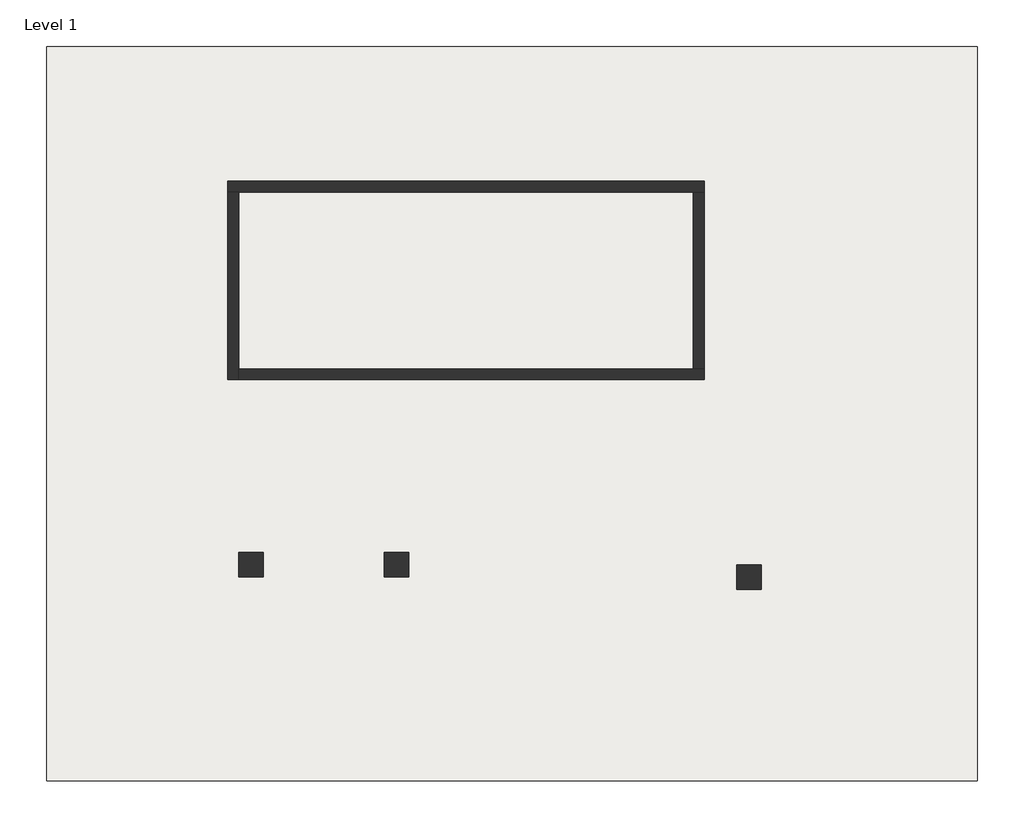
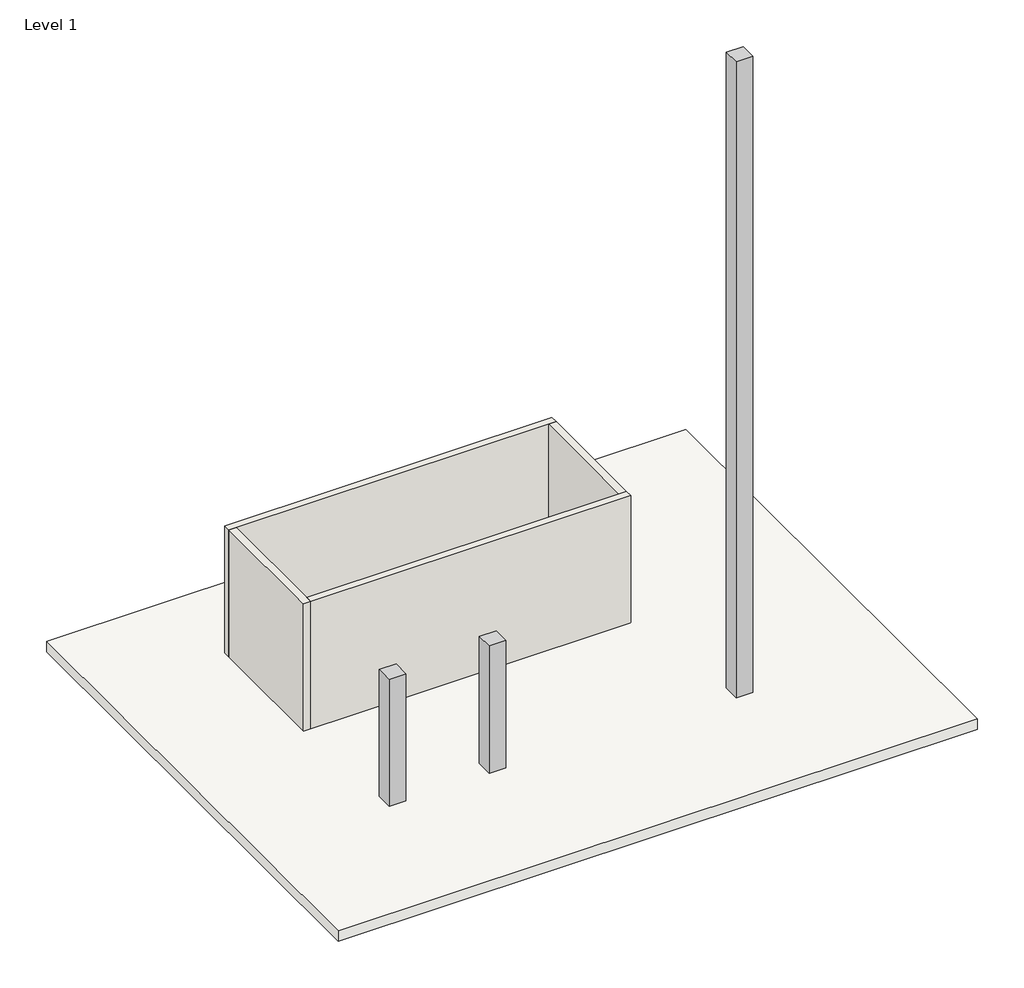
# One storey: 4 walls, 3 columns, 1 slab.
"""IFC4 building model written with IfcOpenShell, lengths in millimetres."""

from ifc_helpers import new_model, si_unit, frame, origin, origin_with_axes, place, context, project, spatial, polyline, outline, extrude, faceted_brep, transform, mapped, element, save
from components import column_ce396696

model = new_model("IFC4")

# Units and contexts
model_context = context("Model", 3, world=origin())
ifc_project = project(units=[si_unit("LENGTHUNIT", "METRE", prefix="MILLI")], contexts=[model_context])

# Site, building, storey
site = spatial("IfcSite", under=ifc_project)
building = spatial("IfcBuilding", under=site)
storey = spatial("IfcBuildingStorey", under=building, Name="Level 1", Elevation=0.0)

# Columns
placement = place(None, origin())
element("IfcColumn", 1, ObjectType="Rectangular Column : 18\" x 18\"", at=placement, inside=storey, context=model_context, shape_type="SweptSolid", body=[
    extrude(outline(polyline([(-3589.1492777, 3617.6297737), (-3589.1492777, 3160.4297737), (-4046.3492777, 3160.4297737), (-4046.3492777, 3617.6297737), (-3589.1492777, 3617.6297737)])), origin_with_axes(), (0.0, 0.0, 1.0), 18288.0),
])
column_shape = column_ce396696(model_context)
element("IfcColumn", 2, ObjectType="Rectangular Column : 18\" x 18\"", at=placement, inside=storey, context=model_context, shape_type="MappedRepresentation", body=[
    mapped(column_shape, transform((-10396.3492777, 3617.6297737, 0.0), x_axis=(1.0, 0.0, 0.0), y_axis=(0.0, 1.0, 0.0), z_axis=(0.0, 0.0, 1.0))),
])
element("IfcColumn", 3, ObjectType="Rectangular Column : 18\" x 18\"", at=placement, inside=storey, context=model_context, shape_type="MappedRepresentation", body=[
    mapped(column_shape, transform((-13114.1492777, 3617.6297737, 0.0), x_axis=(1.0, 0.0, 0.0), y_axis=(0.0, 1.0, 0.0), z_axis=(0.0, 0.0, 1.0))),
])

# Slab
element("IfcSlab", 4, ObjectType="Generic - 12\"", at=placement, inside=storey, context=model_context, shape_type="SweptSolid", body=[
    extrude(outline(polyline([(442.3947155, 13293.9108811), (442.3947155, -422.0891189), (-16931.2052845, -422.0891189), (-16931.2052845, 13293.9108811), (442.3947155, 13293.9108811)])), frame((0.0, 0.0, -304.8), z_axis=(0.0, 0.0, 1.0), x_axis=(1.0, 0.0, 0.0)), (0.0, 0.0, 1.0), 304.8),
])

# Walls
element("IfcWall", 5, ObjectType="Generic - 8\"", at=placement, inside=storey, context=model_context, shape_type="Brep", body=[
    faceted_brep([(-13545.9492777, 10577.2297737, 0.0), (-13342.7492777, 10577.2297737, 0.0), (-4859.1492777, 10577.2297737, 0.0), (-4655.9492777, 10577.2297737, 0.0), (-4655.9492777, 10577.2297737, 3657.6), (-4859.1492777, 10577.2297737, 3657.6), (-13342.7492777, 10577.2297737, 3657.6), (-13545.9492777, 10577.2297737, 3657.6), (-13545.9492777, 10780.4297737, 0.0), (-13545.9492777, 10780.4297737, 3657.6), (-4655.9492777, 10780.4297737, 3657.6), (-4655.9492777, 10780.4297737, 0.0)], [[[0, 1, 2, 3, 4, 5, 6, 7]], [[8, 9, 10, 11]], [[3, 2, 1, 0, 8, 11]], [[7, 6, 5, 4, 10, 9]], [[0, 7, 9, 8]], [[4, 3, 11, 10]]]),
])
element("IfcWall", 6, ObjectType="Generic - 8\"", at=placement, inside=storey, context=model_context, shape_type="Brep", body=[
    faceted_brep([(-13545.9492777, 10577.2297737, 0.0), (-13545.9492777, 7072.0297737, 0.0), (-13545.9492777, 7072.0297737, 3657.6), (-13545.9492777, 10577.2297737, 3657.6), (-13342.7492777, 10577.2297737, 0.0), (-13342.7492777, 10577.2297737, 3657.6), (-13342.7492777, 7275.2297737, 3657.6), (-13342.7492777, 7072.0297737, 3657.6), (-13342.7492777, 7072.0297737, 0.0), (-13342.7492777, 7275.2297737, 0.0)], [[[0, 1, 2, 3]], [[4, 5, 6, 7, 8, 9]], [[1, 0, 4, 9, 8]], [[3, 2, 7, 6, 5]], [[0, 3, 5, 4]], [[2, 1, 8, 7]]]),
])
element("IfcWall", 7, ObjectType="Generic - 8\"", at=placement, inside=storey, context=model_context, shape_type="Brep", body=[
    faceted_brep([(-13342.7492777, 7072.0297737, 0.0), (-4655.9492777, 7072.0297737, 0.0), (-4655.9492777, 7072.0297737, 3657.6), (-13342.7492777, 7072.0297737, 3657.6), (-13342.7492777, 7275.2297737, 0.0), (-13342.7492777, 7275.2297737, 3657.6), (-4859.1492777, 7275.2297737, 3657.6), (-4655.9492777, 7275.2297737, 3657.6), (-4655.9492777, 7275.2297737, 0.0), (-4859.1492777, 7275.2297737, 0.0)], [[[0, 1, 2, 3]], [[4, 5, 6, 7, 8, 9]], [[1, 0, 4, 9, 8]], [[3, 2, 7, 6, 5]], [[0, 3, 5, 4]], [[2, 1, 8, 7]]]),
])
element("IfcWall", 8, ObjectType="Generic - 8\"", at=placement, inside=storey, context=model_context, shape_type="SweptSolid", body=[
    extrude(outline(polyline([(-4655.9492777, 10577.2297737), (-4655.9492777, 7275.2297737), (-4859.1492777, 7275.2297737), (-4859.1492777, 10577.2297737), (-4655.9492777, 10577.2297737)])), origin_with_axes(), (0.0, 0.0, 1.0), 3657.6),
])

save(model, "model.ifc")

# Revit data of these elements
# Type "Rectangular Column : 18\" x 18\""
#   Assembly Code = "B1010200"
#   Depth = 1' - 6"
#   Offset Base = 0' - 0"
#   Offset Top = 0' - 0"
#   Width = 1' - 6"
#   Material = none
# Type "Generic - 12\""
#   Assembly Code = "B1010"
#   Function = 0
#   Layers, outside or top first: 1' - 0" no material (function 1)
# Type "Generic - 8\""
#   Assembly Code = "B2010"
#   Layers, outside or top first: 0' - 8" no material (function 1)
# Elements 1, 2, 3 (IfcColumn, "Rectangular Column : 18\" x 18\"")
#   Phase Created = New Construction
# Element 4 (IfcSlab, "Generic - 12\"")
#   Height Offset From Level = 0' - 0"
#   Phase Created = New Construction
#   Materials on its faces: "Default Floor"
# Elements 5, 6, 7, 8 (IfcWall, "Generic - 8\"")
#   Top Offset = 0' - 0"
#   Base Offset = 0' - 0"
#   Unconnected Height = 12' - 0"
#   wall height = 12' - 0"
#   Phase Created = New Construction
#   Base Constraint = Level 1
#   Materials on its faces: "Default Wall"
# Materials
#   "Default Floor": colour RGB 128 128 128, transparency 0
#   "Default Wall": colour RGB 128 128 128, transparency 0
